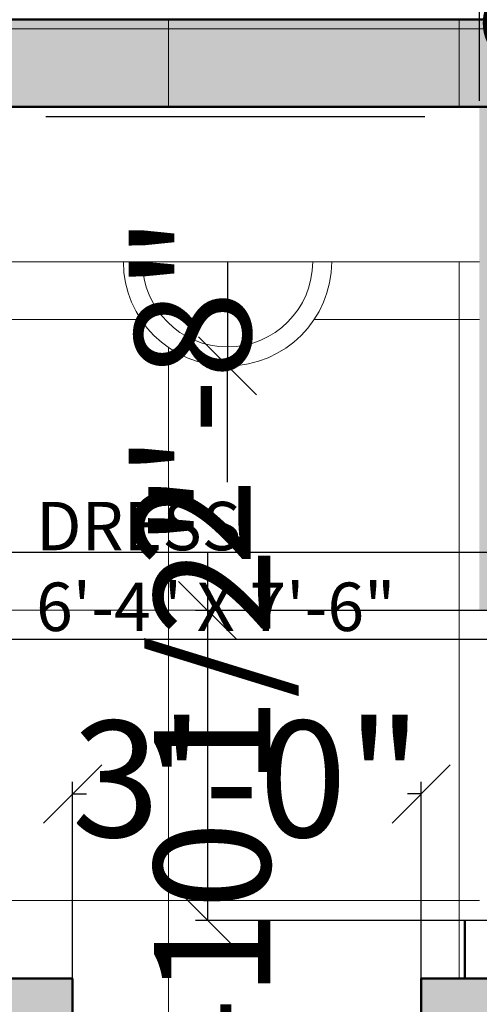
# Model space of a CAD drawing. Units: inches. Extents: x 2371 to 3019, y 129 to 700.
# Tile 5 of 14: x 2445 to 2492, y 529 to 631. Entities that reach past the tile are written whole.
import ezdxf

# ---------------------------------------------------------------- set-up
doc = ezdxf.new("R2010")
doc.units = ezdxf.units.IN
for name, color, linetype, lineweight in [('A-ANNO-DIMS', 2, 'Continuous', 18), ('A-AREA-IDEN', 7, 'Continuous', 25), ('A-DOOR', 4, 'Continuous', 25), ('A-FLOR-FIXT', 8, 'Continuous', 18), ('A-FLOR-PATT', 252, 'Continuous', 13), ('A-FURN', 8, 'Continuous', 18), ('A-GLAZ', 4, 'Continuous', 25), ('A-WALL', 7, 'Continuous', 50), ('A-WALL-PATT', 8, 'Continuous', 13)]:
    doc.layers.add(name, color=color, linetype=linetype, lineweight=lineweight)
doc.styles.get("Standard").update_dxf_attribs({"font": 'arial.ttf'})
doc.dimstyles.new('ISO-25', dxfattribs={"dimtxt": 12, "dimasz": 6, "dimexe": 1.25, "dimexo": 0.625, "dimtad": 0, "dimdec": 1, "dimlunit": 3, "dimtxsty": 'Standard', "dimblk": 'OBLIQUE', "dimblk1": 'ORIGIN2', "dimblk2": 'OBLIQUE', "dimcen": 2.5, "dimadec": 0, "dimazin": 0, "dimtfac": 1, "dimtdec": 1, "dimtmove": 0, "dimatfit": 3, "dimldrblk": 'OBLIQUE', "dimfxl": 1, "dimarcsym": 0})

# ---------------------------------------------------------------- blocks, each defined once
blk = doc.blocks.new('*U3')
for p, q in [((0, 0), (0, -6)), ((-32, 0), (-32, -6))]:
    blk.add_line(p, q)
blk.add_lwpolyline([(0, 0), (-27.71, 16), (-28.59, 14.48), (-0.88, -1.52)], close=True)
blk.add_arc((0, 0), 32, 150, 180)
blk = doc.blocks.new('_Oblique')
at = {"color": 0, "linetype": 'ByBlock', "lineweight": -2}
blk.add_line((-0.5, -0.5), (0.5, 0.5), dxfattribs=at)
blk = doc.blocks.new('*D14')
at = {"layer": 'A-ANNO-DIMS', "color": 0, "lineweight": -2, "transparency": 16777216}
for p, q in [((2407.11, 631.6), (2407.11, 649.37)), ((2923.11, 631.6), (2923.11, 649.37)), ((2407.11, 648.12), (2643.63, 648.12)), ((2923.11, 648.12), (2686.58, 648.12))]:
    blk.add_line(p, q, dxfattribs=at)
at = {"layer": 'Defpoints', "color": 0, "lineweight": 25, "transparency": 16777216}
for p in [(2923.11, 648.12), (2407.11, 630.98), (2923.11, 630.98)]:
    blk.add_point(p, dxfattribs=at)
at = {"layer": 'A-ANNO-DIMS', "color": 0, "lineweight": -2, "transparency": 16777216, "xscale": 6, "yscale": 6, "zscale": 6, "rotation": 180}
blk.add_blockref('_Oblique', (2407.11, 648.12), dxfattribs=at)
at = {"layer": 'A-ANNO-DIMS', "color": 0, "lineweight": -2, "transparency": 16777216, "xscale": 6, "yscale": 6, "zscale": 6}
blk.add_blockref('_Oblique', (2923.11, 648.12), dxfattribs=at)
at = {"layer": 'A-ANNO-DIMS', "color": 0, "transparency": 16777216, "insert": (2665.11, 648.12), "char_height": 12, "width": 20.8486, "attachment_point": 5}
blk.add_mtext('43\'-0"', dxfattribs=at)
blk = doc.blocks.new('_Origin2')
at = {"color": 0, "linetype": 'ByBlock', "lineweight": -2}
blk.add_line((-0.5, 0), (-1, 0), dxfattribs=at)
for radius in [0.5, 0.25]:
    blk.add_circle((0, 0), radius, dxfattribs=at)
blk = doc.blocks.new('*D34')
at = {"layer": 'A-ANNO-DIMS', "color": 0, "lineweight": -2, "transparency": 16777216}
for p, q in [((2407.11, 631.6), (2407.11, 660.28)), ((2416.11, 622.6), (2416.11, 660.28)), ((2407.11, 659.03), (2416.11, 659.03)), ((2416.11, 659.03), (2422.11, 659.03))]:
    blk.add_line(p, q, dxfattribs=at)
at = {"layer": 'Defpoints', "color": 0, "lineweight": 25, "transparency": 16777216}
for p in [(2416.11, 659.03), (2407.11, 630.98), (2416.11, 621.98)]:
    blk.add_point(p, dxfattribs=at)
at = {"layer": 'A-ANNO-DIMS', "color": 0, "lineweight": -2, "transparency": 16777216, "xscale": 6, "yscale": 6, "zscale": 6, "rotation": 180}
blk.add_blockref('_Oblique', (2407.11, 659.03), dxfattribs=at)
at = {"layer": 'A-ANNO-DIMS', "color": 0, "lineweight": -2, "transparency": 16777216, "xscale": 6, "yscale": 6, "zscale": 6}
blk.add_blockref('_Oblique', (2416.11, 659.03), dxfattribs=at)
at = {"layer": 'A-ANNO-DIMS', "color": 0, "transparency": 16777216, "insert": (2438.68, 659.03), "char_height": 12, "attachment_point": 5}
blk.add_mtext('0\'-9"', dxfattribs=at)
blk = doc.blocks.new('*D35')
at = {"layer": 'A-ANNO-DIMS', "color": 0, "lineweight": -2, "transparency": 16777216}
for p, q in [((2416.11, 622.6), (2416.11, 660.28)), ((2492.11, 622.6), (2492.11, 660.28)), ((2416.11, 659.03), (2437.5, 659.03)), ((2492.11, 659.03), (2470.71, 659.03))]:
    blk.add_line(p, q, dxfattribs=at)
at = {"layer": 'Defpoints', "color": 0, "lineweight": 25, "transparency": 16777216}
for p in [(2492.11, 659.03), (2416.11, 621.98), (2492.11, 621.98)]:
    blk.add_point(p, dxfattribs=at)
at = {"layer": 'A-ANNO-DIMS', "color": 0, "lineweight": -2, "transparency": 16777216, "xscale": 6, "yscale": 6, "zscale": 6, "rotation": 180}
blk.add_blockref('_Oblique', (2416.11, 659.03), dxfattribs=at)
at = {"layer": 'A-ANNO-DIMS', "color": 0, "lineweight": -2, "transparency": 16777216, "xscale": 6, "yscale": 6, "zscale": 6}
blk.add_blockref('_Oblique', (2492.11, 659.03), dxfattribs=at)
at = {"layer": 'A-ANNO-DIMS', "color": 0, "transparency": 16777216, "insert": (2454.11, 659.03), "char_height": 12, "attachment_point": 5}
blk.add_mtext('6\'-4"', dxfattribs=at)
blk = doc.blocks.new('*D36')
at = {"layer": 'A-ANNO-DIMS', "color": 0, "lineweight": -2, "transparency": 16777216}
for p, q in [((2492.11, 622.6), (2492.11, 660.28)), ((2496.61, 622.6), (2496.61, 660.28)), ((2492.11, 659.03), (2496.61, 659.03)), ((2496.61, 659.03), (2502.61, 659.03))]:
    blk.add_line(p, q, dxfattribs=at)
at = {"layer": 'Defpoints', "color": 0, "lineweight": 25, "transparency": 16777216}
for p in [(2496.61, 659.03), (2492.11, 621.98), (2496.61, 621.98)]:
    blk.add_point(p, dxfattribs=at)
at = {"layer": 'A-ANNO-DIMS', "color": 0, "lineweight": -2, "transparency": 16777216, "xscale": 6, "yscale": 6, "zscale": 6, "rotation": 180}
blk.add_blockref('_Oblique', (2492.11, 659.03), dxfattribs=at)
at = {"layer": 'A-ANNO-DIMS', "color": 0, "lineweight": -2, "transparency": 16777216, "xscale": 6, "yscale": 6, "zscale": 6}
blk.add_blockref('_Oblique', (2496.61, 659.03), dxfattribs=at)
at = {"layer": 'A-ANNO-DIMS', "color": 0, "transparency": 16777216, "insert": (2533.16, 659.03), "char_height": 12, "attachment_point": 5}
blk.add_mtext('0\'-4 1/2"', dxfattribs=at)
blk = doc.blocks.new('*D65')
at = {"layer": 'A-ANNO-DIMS', "color": 0, "lineweight": -2, "transparency": 16777216}
for p, q in [((2618.98, 621.98), (2377.81, 621.98)), ((2379.06, 621.98), (2379.06, 620.21)), ((2379.06, 575.98), (2379.06, 577.74)), ((2616.98, 575.98), (2377.81, 575.98))]:
    blk.add_line(p, q, dxfattribs=at)
at = {"layer": 'Defpoints', "color": 0, "lineweight": 25, "transparency": 16777216}
for p in [(2379.06, 621.98), (2619.61, 621.98), (2617.61, 575.98)]:
    blk.add_point(p, dxfattribs=at)
at = {"layer": 'A-ANNO-DIMS', "color": 0, "lineweight": -2, "transparency": 16777216, "xscale": 6, "yscale": 6, "zscale": 6}
for p, rotation in [((2379.06, 621.98), 90), ((2379.06, 575.98), 270)]:
    blk.add_blockref('_Oblique', p, dxfattribs=dict(at, rotation=rotation))
at = {"layer": 'A-ANNO-DIMS', "color": 0, "transparency": 16777216, "insert": (2379.06, 598.98), "char_height": 12, "attachment_point": 5, "rotation": 90}
blk.add_mtext('3\'-10"', dxfattribs=at)
blk = doc.blocks.new('*D67')
at = {"layer": 'A-ANNO-DIMS', "color": 0, "lineweight": -2, "transparency": 16777216}
for p, q in [((2379.06, 575.98), (2379.06, 581.98)), ((2616.98, 575.98), (2377.81, 575.98)), ((2379.06, 566.98), (2379.06, 575.98)), ((2616.98, 566.98), (2377.81, 566.98))]:
    blk.add_line(p, q, dxfattribs=at)
at = {"layer": 'Defpoints', "color": 0, "lineweight": 25, "transparency": 16777216}
for p in [(2379.06, 575.98), (2617.61, 575.98), (2617.61, 566.98)]:
    blk.add_point(p, dxfattribs=at)
at = {"layer": 'A-ANNO-DIMS', "color": 0, "lineweight": -2, "transparency": 16777216, "xscale": 6, "yscale": 6, "zscale": 6}
for p, rotation in [((2379.06, 575.98), 90), ((2379.06, 566.98), 270)]:
    blk.add_blockref('_Oblique', p, dxfattribs=dict(at, rotation=rotation))
at = {"layer": 'A-ANNO-DIMS', "color": 0, "transparency": 16777216, "insert": (2379.06, 598.55), "char_height": 12, "attachment_point": 5, "rotation": 90}
blk.add_mtext('0\'-9"', dxfattribs=at)
blk = doc.blocks.new('*D74')
at = {"layer": 'A-ANNO-DIMS', "color": 0, "lineweight": -2, "transparency": 16777216}
for p, q in [((2464.06, 569.98), (2464.06, 575.98)), ((2491.48, 569.98), (2462.81, 569.98)), ((2464.06, 537.98), (2464.06, 569.98)), ((2491.48, 537.98), (2462.81, 537.98))]:
    blk.add_line(p, q, dxfattribs=at)
at = {"layer": 'Defpoints', "color": 0, "lineweight": 25, "transparency": 16777216}
for p in [(2464.06, 569.98), (2492.11, 569.98), (2492.11, 537.98)]:
    blk.add_point(p, dxfattribs=at)
at = {"layer": 'A-ANNO-DIMS', "color": 0, "lineweight": -2, "transparency": 16777216, "xscale": 6, "yscale": 6, "zscale": 6}
for p, rotation in [((2464.06, 569.98), 90), ((2464.06, 537.98), 270)]:
    blk.add_blockref('_Oblique', p, dxfattribs=dict(at, rotation=rotation))
at = {"layer": 'A-ANNO-DIMS', "color": 0, "transparency": 16777216, "insert": (2464.06, 592.65), "char_height": 12, "attachment_point": 5, "rotation": 90}
blk.add_mtext('2\'-8"', dxfattribs=at)
blk = doc.blocks.new('*D76')
at = {"layer": 'A-ANNO-DIMS', "color": 0, "lineweight": -2, "transparency": 16777216}
for p, q in [((2450.11, 523.6), (2450.11, 552.28)), ((2486.11, 523.6), (2486.11, 552.28)), ((2450.11, 551.03), (2451.53, 551.03)), ((2486.11, 551.03), (2484.68, 551.03))]:
    blk.add_line(p, q, dxfattribs=at)
at = {"layer": 'Defpoints', "color": 0, "lineweight": 25, "transparency": 16777216}
for p in [(2486.11, 551.03), (2450.11, 522.98), (2486.11, 522.98)]:
    blk.add_point(p, dxfattribs=at)
at = {"layer": 'A-ANNO-DIMS', "color": 0, "lineweight": -2, "transparency": 16777216, "xscale": 6, "yscale": 6, "zscale": 6, "rotation": 180}
blk.add_blockref('_Oblique', (2450.11, 551.03), dxfattribs=at)
at = {"layer": 'A-ANNO-DIMS', "color": 0, "lineweight": -2, "transparency": 16777216, "xscale": 6, "yscale": 6, "zscale": 6}
blk.add_blockref('_Oblique', (2486.11, 551.03), dxfattribs=at)
at = {"layer": 'A-ANNO-DIMS', "color": 0, "transparency": 16777216, "insert": (2468.11, 551.03), "char_height": 12, "attachment_point": 5}
blk.add_mtext('3\'-0"', dxfattribs=at)
blk = doc.blocks.new('*D78')
at = {"layer": 'A-ANNO-DIMS', "color": 0, "lineweight": -2, "transparency": 16777216}
for p, q in [((2500.23, 621.98), (2500.23, 627.98)), ((2527.66, 621.98), (2498.98, 621.98)), ((2500.23, 580.36), (2500.23, 621.98)), ((2527.66, 580.36), (2498.98, 580.36))]:
    blk.add_line(p, q, dxfattribs=at)
at = {"layer": 'Defpoints', "color": 0, "lineweight": 25, "transparency": 16777216}
for p in [(2500.23, 621.98), (2528.28, 621.98), (2528.28, 580.36)]:
    blk.add_point(p, dxfattribs=at)
at = {"layer": 'A-ANNO-DIMS', "color": 0, "lineweight": -2, "transparency": 16777216, "xscale": 6, "yscale": 6, "zscale": 6}
for p, rotation in [((2500.23, 621.98), 90), ((2500.23, 580.36), 270)]:
    blk.add_blockref('_Oblique', p, dxfattribs=dict(at, rotation=rotation))
at = {"layer": 'A-ANNO-DIMS', "color": 0, "transparency": 16777216, "insert": (2500.23, 658.53), "char_height": 12, "attachment_point": 5, "rotation": 90}
blk.add_mtext('3\'-5 1/2"', dxfattribs=at)
blk = doc.blocks.new('*D81')
at = {"layer": 'A-ANNO-DIMS', "color": 0, "lineweight": -2, "transparency": 16777216}
for p in [(2466.11, 605.98), (2466.09, 583.23)]:
    blk.add_line(p, (2466.1, 595.23), dxfattribs=at)
at = {"layer": 'Defpoints', "color": 0, "lineweight": 25, "transparency": 16777216}
for p in [(2466.11, 605.98), (2466.1, 595.23)]:
    blk.add_point(p, dxfattribs=at)
at = {"layer": 'A-ANNO-DIMS', "color": 0, "lineweight": -2, "transparency": 16777216, "xscale": 6, "yscale": 6, "zscale": 6, "rotation": 89.97280933984025}
blk.add_blockref('_Oblique', (2466.1, 595.23), dxfattribs=at)
at = {"layer": 'A-ANNO-DIMS', "color": 0, "transparency": 16777216, "insert": (2466.07, 542.27), "char_height": 12, "attachment_point": 5, "rotation": 89.9728}
blk.add_mtext('R0\'-10 1/2"', dxfattribs=at)

msp = doc.modelspace()

# ---------------------------------------------------------------- hatches: boundary and pattern name
at = {"layer": 'A-FLOR-PATT'}
h = msp.add_hatch(dxfattribs=at)
h.set_pattern_fill('_USER', color=256, scale=30, pattern_type=0)
h.set_pattern_definition([(0, (0, 0), (0, 30), [])])
h.paths.add_polyline_path([(2913.11, 498.98), (2827.61, 498.98), (2827.61, 531.98), (2832.11, 531.98), (2832.11, 537.98), (2833.61, 537.98), (2833.61, 605.98), (2818.35, 605.98, -1), (2796.86, 605.98), (2781.61, 605.98), (2781.61, 603.98), (2781.61, 533.98), (2757.61, 533.98), (2757.61, 531.98), (2797.61, 531.98), (2797.61, 522.98), (2757.61, 522.98), (2757.61, 516.98), (2754.59, 516.98), (2772.52, 485.76), (2771.01, 484.89), (2770.98, 484.93, -0.097552), (2757.61, 481.1), (2757.61, 422.48), (2837.61, 422.48), (2837.61, 362.48), (2757.61, 362.48), (2757.61, 303.98), (2835.86, 303.98, -0.09439), (2793.86, 311.98), (2793.86, 337.98), (2799.86, 337.98), (2799.86, 336.42), (2871.86, 336.42), (2871.86, 337.98), (2877.86, 337.98), (2877.86, 311.98, -0.09439), (2835.86, 303.98), (2913.11, 303.98), (2913.11, 383.18), (2904.11, 383.18), (2904.11, 419.18), (2913.11, 419.18)])
h.paths.add_polyline_path([(2788.88, 332.88), (2788.88, 308.88), (2764.88, 308.88), (2764.88, 332.88)], flags=16)
h.paths.add_polyline_path([(2788.4, 325.04, -1), (2774.4, 325.04, -1)], flags=0)
h.paths.add_polyline_path([(2781.4, 328.04), (2784.4, 325.04), (2781.4, 322.04), (2778.4, 325.04)], flags=0)
h.paths.add_polyline_path([(2782.4, 325.04, -1), (2780.4, 325.04, -1)], flags=0)
h.paths.add_polyline_path([(2748.61, 480.99), (2754.51, 480.98, 0.119303), (2770.98, 484.93), (2753.07, 516.1), (2754.59, 516.98), (2748.61, 516.98), (2748.61, 539.98), (2712.61, 539.98), (2665.11, 539.98, -0.09439), (2707.11, 531.98), (2707.11, 505.98), (2701.11, 505.98), (2701.11, 507.53), (2629.11, 507.53), (2629.11, 505.98), (2623.11, 505.98), (2623.11, 531.98, -0.09439), (2665.11, 539.98), (2581.61, 539.98), (2581.61, 522.98), (2581.61, 477.98, -0.131044), (2589.61, 507.98), (2615.61, 507.98), (2615.61, 501.98), (2614.05, 501.98), (2614.05, 453.98), (2615.61, 453.98), (2615.61, 447.98), (2589.61, 447.98, -0.131044), (2581.61, 477.98), (2581.61, 432.98), (2572.61, 432.98, 0.119303), (2556.14, 428.99), (2574.12, 397.85), (2572.61, 396.98), (2578.61, 396.98), (2581.61, 396.98), (2581.61, 390.98), (2748.61, 390.98)])
h.paths.add_polyline_path([(2683.1, 447.25), (2652.43, 447.25), (2652.43, 492.22), (2683.1, 492.22)], flags=16)
h.paths.add_polyline_path([(2682.1, 448.25), (2653.43, 448.25), (2653.43, 491.22), (2682.1, 491.22)], flags=0)
h.paths.add_polyline_path([(2613.58, 512.06), (2589.58, 512.06), (2589.58, 536.06), (2613.58, 536.06)], flags=16)
h.paths.add_polyline_path([(2599.1, 528.22, -1), (2613.1, 528.22, -1)], flags=0)
h.paths.add_polyline_path([(2609.1, 528.22), (2606.1, 525.22), (2603.1, 528.22), (2606.1, 531.22)], flags=0)
h.paths.add_polyline_path([(2607.1, 528.22, -1), (2605.1, 528.22, -1)], flags=0)
h.paths.add_polyline_path([(2581.61, 522.98), (2581.61, 621.98), (2572.61, 621.98), (2572.61, 522.98), (2572.61, 500.98), (2565.85, 500.98), (2565.85, 500.15), (2564.82, 500.15), (2561.16, 500.19), (2561.16, 500.17), (2560.13, 500.3), (2560.22, 500.98), (2556.38, 500.98), (2556.43, 500.22), (2555.4, 500.14), (2555.34, 500.98), (2551.07, 500.98), (2551.07, 500.15), (2550.04, 500.15), (2547.64, 500.19), (2547.64, 500.15), (2546.61, 500.15), (2541.79, 500.22), (2540.72, 500.13), (2540.65, 500.98), (2533.37, 500.98), (2533.37, 500.15), (2532.34, 500.15), (2529.13, 500.21), (2529.12, 500.13), (2528.09, 500.22), (2528.16, 500.98), (2523.23, 500.98), (2523.23, 500.15), (2522.2, 500.15), (2519.8, 500.21), (2519.8, 500.15), (2518.77, 500.15), (2514.45, 500.26), (2514.44, 500.14), (2513.41, 500.22), (2513.47, 500.98), (2509.62, 500.98), (2509.71, 500.3), (2508.69, 500.17), (2508.58, 500.98), (2505.03, 500.98), (2505.03, 500.15), (2503.99, 500.15), (2501.07, 500.29), (2501.07, 500.15), (2500.04, 500.15), (2496.44, 500.37), (2496.44, 500.15), (2495.4, 500.15), (2492.55, 500.41), (2492.18, 500.35), (2492.09, 500.98), (2486.11, 500.98), (2486.11, 524.98), (2486.11, 531.98), (2490.61, 531.98), (2490.61, 537.98), (2492.11, 537.98), (2492.11, 605.98), (2476.85, 605.98, -1), (2455.36, 605.98), (2440.11, 605.98), (2440.11, 533.98), (2416.11, 533.98), (2416.11, 605.98), (2416.11, 621.98), (2536.61, 621.98), (2536.61, 630.98), (2407.11, 630.98), (2407.11, 363.98), (2416.11, 363.98), (2416.11, 431.48), (2496.11, 431.48), (2496.11, 371.48), (2416.11, 371.48), (2416.11, 303.98), (2494.36, 303.98, -0.09439), (2452.36, 311.98), (2452.36, 337.98), (2458.36, 337.98), (2458.36, 336.42), (2530.36, 336.42), (2530.36, 337.98), (2536.36, 337.98), (2536.36, 311.98, -0.09439), (2494.36, 303.98), (2572.61, 303.98), (2572.61, 381.98), (2572.61, 396.98), (2554.61, 428.15), (2556.12, 429.03), (2556.14, 428.99, -0.119303), (2572.61, 432.98), (2578.61, 432.98), (2581.61, 432.98)])
h.paths.add_polyline_path([(2450.11, 500.98), (2444.5, 500.98), (2444.44, 500.14), (2443.41, 500.22), (2443.47, 500.98), (2439.62, 500.98), (2439.71, 500.3), (2438.69, 500.17), (2438.58, 500.98), (2435.02, 500.98), (2435.02, 500.15), (2433.99, 500.15), (2433.99, 500.98), (2431.07, 500.98), (2431.07, 500.15), (2430.04, 500.15), (2430.04, 500.98), (2426.43, 500.98), (2426.43, 500.15), (2425.4, 500.15), (2425.4, 500.98), (2423.13, 500.98), (2423.2, 500.5), (2422.18, 500.35), (2422.09, 500.98), (2416.11, 500.98), (2416.11, 524.98), (2416.11, 531.98), (2450.11, 531.98), (2450.11, 522.98)], flags=16)
h.paths.add_polyline_path([(2449.11, 501.98), (2417.11, 501.98), (2417.11, 522.98), (2417.11, 523.98), (2449.11, 523.98)], flags=0)
h.paths.add_polyline_path([(2420.7, 510.73), (2419.36, 520.07), (2420.38, 520.22), (2421.74, 510.73), (2425.4, 510.73), (2425.4, 520.07), (2426.43, 520.07), (2426.43, 510.73), (2430.04, 510.73), (2430.04, 520.07), (2431.07, 520.07), (2431.07, 510.73), (2433.99, 510.73), (2433.99, 520.07), (2435.02, 520.07), (2435.02, 510.73), (2437.35, 510.73), (2436.18, 519.93), (2437.2, 520.06), (2438.39, 510.73), (2444.17, 510.73), (2444.85, 520.08), (2445.88, 520.01), (2445.21, 510.73)], flags=0)
h.paths.add_polyline_path([(2446.94, 336.11), (2446.94, 312.11), (2422.94, 312.11), (2422.94, 336.11)], flags=16)
h.paths.add_polyline_path([(2446.46, 328.27, -1), (2432.46, 328.27, -1)], flags=0)
h.paths.add_polyline_path([(2439.46, 331.27), (2442.46, 328.27), (2439.46, 325.27), (2436.46, 328.27)], flags=0)
h.paths.add_polyline_path([(2440.46, 328.27, -1), (2438.46, 328.27, -1)], flags=0)
h.paths.add_polyline_path([(2816, 444.88), (2866.87, 444.88), (2866.87, 463.54), (2816, 463.54)], flags=24)
h.paths.add_polyline_path([(2794.21, 558.3), (2833.34, 558.3), (2833.34, 576.96), (2794.21, 576.96)], flags=24)
h.paths.add_polyline_path([(2651.69, 411.53), (2711.04, 411.53), (2711.04, 430.19), (2651.69, 430.19)], flags=24)
h.paths.add_polyline_path([(2494.09, 444.88), (2544.97, 444.88), (2544.97, 463.54), (2494.09, 463.54)], flags=24)
h.paths.add_polyline_path([(2444.55, 565.02), (2483.69, 565.02), (2483.69, 583.68), (2444.55, 583.68)], flags=24)
h = msp.add_hatch(dxfattribs=at)
h.set_pattern_fill('_USER', color=256, scale=30, angle=90, pattern_type=0)
h.set_pattern_definition([(90, (0, 0), (-30, 2e-15), [])])
h.paths.add_polyline_path([(2913.11, 498.98), (2827.61, 498.98), (2827.61, 531.98), (2832.11, 531.98), (2832.11, 537.98), (2833.61, 537.98), (2833.61, 605.98), (2818.35, 605.98, -1), (2796.86, 605.98), (2781.61, 605.98), (2781.61, 603.98), (2781.61, 533.98), (2757.61, 533.98), (2757.61, 531.98), (2797.61, 531.98), (2797.61, 522.98), (2757.61, 522.98), (2757.61, 516.98), (2754.59, 516.98), (2772.52, 485.76), (2771.01, 484.89), (2770.98, 484.93, -0.097552), (2757.61, 481.1), (2757.61, 422.48), (2837.61, 422.48), (2837.61, 362.48), (2757.61, 362.48), (2757.61, 303.98), (2835.86, 303.98, -0.09439), (2793.86, 311.98), (2793.86, 337.98), (2799.86, 337.98), (2799.86, 336.42), (2871.86, 336.42), (2871.86, 337.98), (2877.86, 337.98), (2877.86, 311.98, -0.09439), (2835.86, 303.98), (2913.11, 303.98), (2913.11, 383.18), (2904.11, 383.18), (2904.11, 419.18), (2913.11, 419.18)])
h.paths.add_polyline_path([(2788.88, 332.88), (2788.88, 308.88), (2764.88, 308.88), (2764.88, 332.88)], flags=16)
h.paths.add_polyline_path([(2788.4, 325.04, -1), (2774.4, 325.04, -1)], flags=0)
h.paths.add_polyline_path([(2781.4, 328.04), (2784.4, 325.04), (2781.4, 322.04), (2778.4, 325.04)], flags=0)
h.paths.add_polyline_path([(2782.4, 325.04, -1), (2780.4, 325.04, -1)], flags=0)
h.paths.add_polyline_path([(2748.61, 480.99), (2754.51, 480.98, 0.119303), (2770.98, 484.93), (2753.07, 516.1), (2754.59, 516.98), (2748.61, 516.98), (2748.61, 539.98), (2712.61, 539.98), (2665.11, 539.98, -0.09439), (2707.11, 531.98), (2707.11, 505.98), (2701.11, 505.98), (2701.11, 507.53), (2629.11, 507.53), (2629.11, 505.98), (2623.11, 505.98), (2623.11, 531.98, -0.09439), (2665.11, 539.98), (2581.61, 539.98), (2581.61, 522.98), (2581.61, 477.98, -0.131044), (2589.61, 507.98), (2615.61, 507.98), (2615.61, 501.98), (2614.05, 501.98), (2614.05, 453.98), (2615.61, 453.98), (2615.61, 447.98), (2589.61, 447.98, -0.131044), (2581.61, 477.98), (2581.61, 432.98), (2572.61, 432.98, 0.119303), (2556.14, 428.99), (2574.12, 397.85), (2572.61, 396.98), (2578.61, 396.98), (2581.61, 396.98), (2581.61, 390.98), (2748.61, 390.98)])
h.paths.add_polyline_path([(2683.1, 447.25), (2652.43, 447.25), (2652.43, 492.22), (2683.1, 492.22)], flags=16)
h.paths.add_polyline_path([(2682.1, 448.25), (2653.43, 448.25), (2653.43, 491.22), (2682.1, 491.22)], flags=0)
h.paths.add_polyline_path([(2613.58, 512.06), (2589.58, 512.06), (2589.58, 536.06), (2613.58, 536.06)], flags=16)
h.paths.add_polyline_path([(2599.1, 528.22, -1), (2613.1, 528.22, -1)], flags=0)
h.paths.add_polyline_path([(2609.1, 528.22), (2606.1, 525.22), (2603.1, 528.22), (2606.1, 531.22)], flags=0)
h.paths.add_polyline_path([(2607.1, 528.22, -1), (2605.1, 528.22, -1)], flags=0)
h.paths.add_polyline_path([(2581.61, 522.98), (2581.61, 621.98), (2572.61, 621.98), (2572.61, 522.98), (2572.61, 500.98), (2565.85, 500.98), (2565.85, 500.15), (2564.82, 500.15), (2561.16, 500.19), (2561.16, 500.17), (2560.13, 500.3), (2560.22, 500.98), (2556.38, 500.98), (2556.43, 500.22), (2555.4, 500.14), (2555.34, 500.98), (2551.07, 500.98), (2551.07, 500.15), (2550.04, 500.15), (2547.64, 500.19), (2547.64, 500.15), (2546.61, 500.15), (2541.79, 500.22), (2540.72, 500.13), (2540.65, 500.98), (2533.37, 500.98), (2533.37, 500.15), (2532.34, 500.15), (2529.13, 500.21), (2529.12, 500.13), (2528.09, 500.22), (2528.16, 500.98), (2523.23, 500.98), (2523.23, 500.15), (2522.2, 500.15), (2519.8, 500.21), (2519.8, 500.15), (2518.77, 500.15), (2514.45, 500.26), (2514.44, 500.14), (2513.41, 500.22), (2513.47, 500.98), (2509.62, 500.98), (2509.71, 500.3), (2508.69, 500.17), (2508.58, 500.98), (2505.03, 500.98), (2505.03, 500.15), (2503.99, 500.15), (2501.07, 500.29), (2501.07, 500.15), (2500.04, 500.15), (2496.44, 500.37), (2496.44, 500.15), (2495.4, 500.15), (2492.55, 500.41), (2492.18, 500.35), (2492.09, 500.98), (2486.11, 500.98), (2486.11, 524.98), (2486.11, 531.98), (2490.61, 531.98), (2490.61, 537.98), (2492.11, 537.98), (2492.11, 605.98), (2476.85, 605.98, -1), (2455.36, 605.98), (2440.11, 605.98), (2440.11, 533.98), (2416.11, 533.98), (2416.11, 605.98), (2416.11, 621.98), (2536.61, 621.98), (2536.61, 630.98), (2407.11, 630.98), (2407.11, 363.98), (2416.11, 363.98), (2416.11, 431.48), (2496.11, 431.48), (2496.11, 371.48), (2416.11, 371.48), (2416.11, 303.98), (2494.36, 303.98, -0.09439), (2452.36, 311.98), (2452.36, 337.98), (2458.36, 337.98), (2458.36, 336.42), (2530.36, 336.42), (2530.36, 337.98), (2536.36, 337.98), (2536.36, 311.98, -0.09439), (2494.36, 303.98), (2572.61, 303.98), (2572.61, 381.98), (2572.61, 396.98), (2554.61, 428.15), (2556.12, 429.03), (2556.14, 428.99, -0.119303), (2572.61, 432.98), (2578.61, 432.98), (2581.61, 432.98)])
h.paths.add_polyline_path([(2450.11, 500.98), (2444.5, 500.98), (2444.44, 500.14), (2443.41, 500.22), (2443.47, 500.98), (2439.62, 500.98), (2439.71, 500.3), (2438.69, 500.17), (2438.58, 500.98), (2435.02, 500.98), (2435.02, 500.15), (2433.99, 500.15), (2433.99, 500.98), (2431.07, 500.98), (2431.07, 500.15), (2430.04, 500.15), (2430.04, 500.98), (2426.43, 500.98), (2426.43, 500.15), (2425.4, 500.15), (2425.4, 500.98), (2423.13, 500.98), (2423.2, 500.5), (2422.18, 500.35), (2422.09, 500.98), (2416.11, 500.98), (2416.11, 524.98), (2416.11, 531.98), (2450.11, 531.98), (2450.11, 522.98)], flags=16)
h.paths.add_polyline_path([(2449.11, 501.98), (2417.11, 501.98), (2417.11, 522.98), (2417.11, 523.98), (2449.11, 523.98)], flags=0)
h.paths.add_polyline_path([(2420.7, 510.73), (2419.36, 520.07), (2420.38, 520.22), (2421.74, 510.73), (2425.4, 510.73), (2425.4, 520.07), (2426.43, 520.07), (2426.43, 510.73), (2430.04, 510.73), (2430.04, 520.07), (2431.07, 520.07), (2431.07, 510.73), (2433.99, 510.73), (2433.99, 520.07), (2435.02, 520.07), (2435.02, 510.73), (2437.35, 510.73), (2436.18, 519.93), (2437.2, 520.06), (2438.39, 510.73), (2444.17, 510.73), (2444.85, 520.08), (2445.88, 520.01), (2445.21, 510.73)], flags=0)
h.paths.add_polyline_path([(2446.94, 336.11), (2446.94, 312.11), (2422.94, 312.11), (2422.94, 336.11)], flags=16)
h.paths.add_polyline_path([(2446.46, 328.27, -1), (2432.46, 328.27, -1)], flags=0)
h.paths.add_polyline_path([(2439.46, 331.27), (2442.46, 328.27), (2439.46, 325.27), (2436.46, 328.27)], flags=0)
h.paths.add_polyline_path([(2440.46, 328.27, -1), (2438.46, 328.27, -1)], flags=0)
h.paths.add_polyline_path([(2816, 444.88), (2866.87, 444.88), (2866.87, 463.54), (2816, 463.54)], flags=24)
h.paths.add_polyline_path([(2794.21, 558.3), (2833.34, 558.3), (2833.34, 576.96), (2794.21, 576.96)], flags=24)
h.paths.add_polyline_path([(2651.69, 411.53), (2711.04, 411.53), (2711.04, 430.19), (2651.69, 430.19)], flags=24)
h.paths.add_polyline_path([(2494.09, 444.88), (2544.97, 444.88), (2544.97, 463.54), (2494.09, 463.54)], flags=24)
h.paths.add_polyline_path([(2444.55, 565.02), (2483.69, 565.02), (2483.69, 583.68), (2444.55, 583.68)], flags=24)
at = {"layer": 'A-WALL-PATT'}
h = msp.add_hatch(color=256, dxfattribs=at)
h.dxf.hatch_style = 1
h.paths.add_polyline_path([(2536.61, 630.98), (2407.11, 630.98), (2407.11, 363.98), (2416.11, 363.98), (2416.11, 498.98), (2416.11, 522.98), (2416.11, 531.98), (2416.11, 603.98), (2416.11, 621.98), (2536.61, 621.98)])
h.paths.add_polyline_path([(2630.98, 630.98), (2560.61, 630.98), (2560.61, 621.98), (2630.98, 621.98)])
h.paths.add_polyline_path([(2878.11, 630.98), (2699.23, 630.98), (2699.23, 621.98), (2878.11, 621.98)])
h.paths.add_polyline_path([(2496.61, 621.98), (2492.11, 621.98), (2492.11, 569.98), (2496.61, 569.98)], flags=17)
h.paths.add_polyline_path([(2581.61, 621.98), (2572.61, 621.98), (2572.61, 522.98), (2572.61, 498.98), (2572.61, 432.98), (2578.61, 432.98), (2581.61, 432.98), (2581.61, 522.98)])
h.paths.add_polyline_path([(2572.61, 531.98), (2486.11, 531.98), (2486.11, 522.98), (2572.61, 522.98)])
h.paths.add_polyline_path([(2450.11, 531.98), (2440.11, 531.98), (2416.11, 531.98), (2416.11, 522.98), (2450.11, 522.98)], flags=17)
h.paths.add_polyline_path([(2416.11, 315.98), (2407.11, 315.98), (2407.11, 294.98), (2458.11, 294.98), (2458.11, 303.98), (2416.11, 303.98)])
h.paths.add_polyline_path([(2757.61, 303.98), (2530.61, 303.98), (2530.61, 294.98), (2757.61, 294.98)])
h.paths.add_polyline_path([(2581.61, 381.98), (2605.61, 381.98), (2617.61, 381.98), (2617.61, 390.98), (2581.61, 390.98), (2581.61, 396.98), (2572.61, 396.98), (2572.61, 381.98), (2572.61, 303.98), (2581.61, 303.98)])
h.paths.add_polyline_path([(2757.61, 480.98), (2748.61, 480.98), (2748.61, 381.98), (2748.61, 303.98), (2757.61, 303.98), (2757.61, 381.98), (2757.61, 422.48)])
h.paths.add_polyline_path([(2797.61, 531.98), (2757.61, 531.98), (2757.61, 603.98), (2757.61, 621.98), (2748.61, 621.98), (2748.61, 516.99), (2754.59, 516.98), (2757.61, 516.98), (2757.61, 522.98), (2797.61, 522.98)])
h.paths.add_polyline_path([(2913.11, 531.98), (2827.61, 531.98), (2827.61, 522.98), (2913.11, 522.98)])
h.paths.add_polyline_path([(2923.11, 630.98), (2902.11, 630.98), (2902.11, 621.98), (2914.11, 621.98), (2914.11, 363.98), (2923.11, 363.98)])
h.paths.add_polyline_path([(2923.11, 315.98), (2914.11, 315.98), (2914.11, 303.98), (2866.11, 303.98), (2866.11, 294.98), (2923.11, 294.98)])
h.paths.add_polyline_path([(2793.61, 303.98), (2757.61, 303.98), (2757.61, 294.98), (2793.61, 294.98)])

# ---------------------------------------------------------------- linework, layer by layer
at = {"layer": 'A-FLOR-FIXT'}
for radius in [10.75, 8.79]:
    msp.add_arc((2466.11, 605.98), radius, 180, 0, dxfattribs=at)
at = {"layer": 'A-FURN'}
msp.add_line((2492.11, 605.98), (2440.11, 605.98), dxfattribs=at)
at = {"layer": 'A-GLAZ'}
msp.add_line((2447.33, 620.98), (2486.47, 620.98), dxfattribs=at)
at = {"layer": 'A-WALL'}
for p, q in [((2536.61, 630.98), (2407.11, 630.98)), ((2536.61, 621.98), (2416.11, 621.98)), ((2490.61, 537.98), (2490.61, 531.98)), ((2450.11, 531.98), (2416.11, 531.98)), ((2450.11, 531.98), (2450.11, 522.98)), ((2572.61, 531.98), (2486.11, 531.98)), ((2486.11, 531.98), (2486.11, 522.98))]:
    msp.add_line(p, q, dxfattribs=at)

# ---------------------------------------------------------------- block references
at = {"layer": 'A-DOOR', "rotation": 270}
msp.add_blockref('*U3', (2496.61, 537.98), dxfattribs=at)

# ---------------------------------------------------------------- texts
at = {"layer": 'A-AREA-IDEN', "ltscale": 2, "insert": (2446.34, 581.19), "char_height": 5, "attachment_point": 1}
msp.add_mtext_dynamic_manual_height_columns('DRESS\\P6\'-4" X 7\'-6"', width=39.2097, gutter_width=12.5, heights=[0], dxfattribs=at)

# ---------------------------------------------------------------- dimensions: what is measured, and where the dimension line sits
at = {"layer": 'A-ANNO-DIMS'}
for base, p1, p2, picture, middle in [((2500.23, 621.98), (2528.28, 580.36), (2528.28, 621.98), '*D78', (2500.23, 658.53)), ((2379.06, 621.98), (2617.61, 575.98), (2619.61, 621.98), '*D65', (2379.06, 598.98)), ((2379.06, 575.98), (2617.61, 566.98), (2617.61, 575.98), '*D67', (2379.06, 598.55)), ((2464.06, 569.98), (2492.11, 537.98), (2492.11, 569.98), '*D74', (2464.06, 592.65))]:
    dim = msp.add_linear_dim(base=base, p1=p1, p2=p2, angle=90, dimstyle='ISO-25', override={"dimdec": 1, "dimlfac": 1, "dimrnd": 0, "dimzin": 1, "dimdsep": 46, "dimlunit": 4, "dimfrac": 2}, dxfattribs=at)
    dim.commit()
    dim.dimension.update_dxf_attribs({"geometry": picture, "text_midpoint": middle})
for base, p1, p2, picture, middle in [((2496.61, 659.03), (2492.11, 621.98), (2496.61, 621.98), '*D36', (2533.16, 659.03)), ((2416.11, 659.03), (2407.11, 630.98), (2416.11, 621.98), '*D34', (2438.68, 659.03)), ((2492.11, 659.03), (2416.11, 621.98), (2492.11, 621.98), '*D35', (2454.11, 659.03)), ((2486.11, 551.03), (2450.11, 522.98), (2486.11, 522.98), '*D76', (2468.11, 551.03))]:
    dim = msp.add_linear_dim(base=base, p1=p1, p2=p2, dimstyle='ISO-25', override={"dimdec": 1, "dimlfac": 1, "dimrnd": 0, "dimzin": 1, "dimdsep": 46, "dimlunit": 4, "dimfrac": 2}, dxfattribs=at)
    dim.commit()
    dim.dimension.update_dxf_attribs({"geometry": picture, "text_midpoint": middle})
dim = msp.add_linear_dim(base=(2923.11, 648.12), p1=(2407.11, 630.98), p2=(2923.11, 630.98), text='43\'-0"', dimstyle='ISO-25', override={"dimclrd": 0, "dimclre": 0, "dimclrt": 0}, dxfattribs=at)
dim.commit()
dim.dimension.update_dxf_attribs({"geometry": '*D14', "text_midpoint": (2665.11, 648.12)})
dim = msp.add_radius_dim(center=(2466.1051, 605.9762), mpoint=(2466.1, 595.2295), dimstyle='ISO-25', override={"dimdec": 1, "dimlfac": 1, "dimrnd": 0, "dimzin": 1, "dimdsep": 46, "dimlunit": 4, "dimfrac": 2}, dxfattribs=at)
dim.commit()
dim.dimension.update_dxf_attribs({"geometry": '*D81', "text_midpoint": (2466.0749, 542.2703)})

doc.saveas('drawing.dxf')
